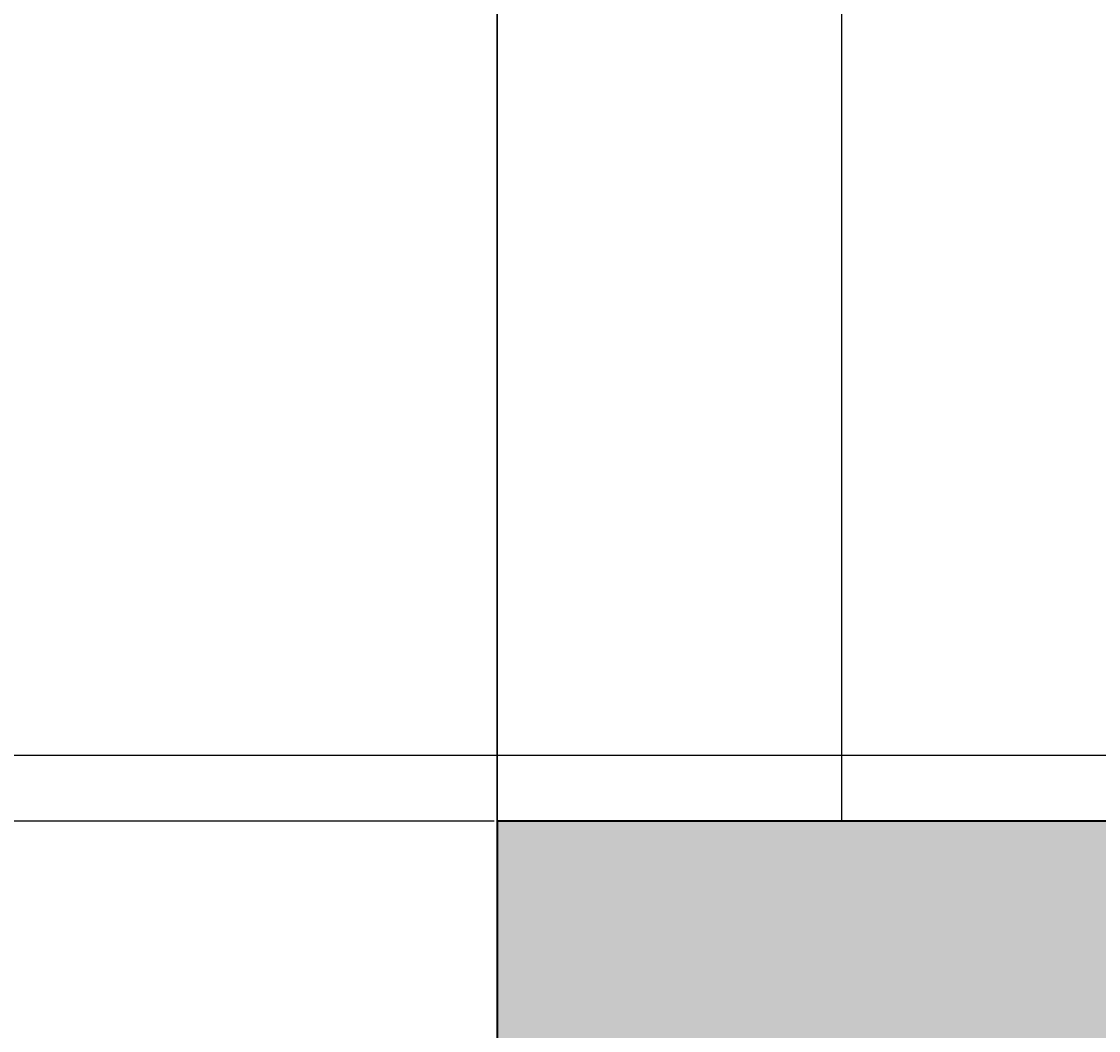
# Model space of a CAD drawing. Units: inches. Extents: x 1998 to 2588, y 1139 to 1977.
# Tile 105 of 134: x 2397 to 2422, y 1590 to 1613. Entities that reach past the tile are written whole.
import ezdxf

# ---------------------------------------------------------------- set-up
doc = ezdxf.new("R2010")
doc.units = ezdxf.units.IN
for name, color, linetype, lineweight in [('A-ANNO-DIMS', 2, 'Continuous', 18), ('A-FLOR-EVTR', 7, 'Continuous', 35), ('A-FLOR-STRS', 7, 'Continuous', 25), ('A-WALL-PATT', 252, 'Continuous', 13)]:
    doc.layers.add(name, color=color, linetype=linetype, lineweight=lineweight)
doc.styles.get("Standard").update_dxf_attribs({"font": 'arial.ttf'})
doc.dimstyles.get("Standard").update_dxf_attribs({"dimtxt": 0.18, "dimasz": 0.18, "dimexe": 0.18, "dimexo": 0.0625, "dimgap": 0.09, "dimtad": 0, "dimtih": 1, "dimtoh": 1, "dimdec": 4, "dimzin": 0, "dimdsep": 46, "dimtxsty": 'Standard', "dimcen": 0.09, "dimadec": 0, "dimazin": 0, "dimtfac": 1, "dimtdec": 4, "dimtofl": 0, "dimtmove": 0, "dimatfit": 3, "dimfxl": 1, "dimtolj": 1, "dimtzin": 0, "dimarcsym": 0})

# ---------------------------------------------------------------- blocks, each defined once
blk = doc.blocks.new('*D24')
at = {"layer": 'A-ANNO-DIMS', "color": 0, "lineweight": -2, "transparency": 16777216}
for p, q in [((2398.535, 1911.232), (2588.309, 1911.232)), ((2588.129, 1911.052), (2588.129, 1570.164)), ((2588.129, 1228.912), (2588.129, 1569.8)), ((2527.535, 1228.732), (2588.309, 1228.732))]:
    blk.add_line(p, q, dxfattribs=at)
at = {"layer": 'A-ANNO-DIMS', "color": 0, "transparency": 16777216}
for points in [[(2588.099, 1911.052), (2588.159, 1911.052), (2588.129, 1911.232)], [(2588.099, 1228.912), (2588.159, 1228.912), (2588.129, 1228.732)]]:
    blk.add_solid(points, dxfattribs=at)
at = {"layer": 'Defpoints', "color": 0, "transparency": 16777216}
for p in [(2398.473, 1911.232), (2588.129, 1911.232), (2527.473, 1228.732)]:
    blk.add_point(p, dxfattribs=at)
at = {"layer": 'A-ANNO-DIMS', "color": 0, "transparency": 16777216, "insert": (2588.129, 1569.982), "char_height": 0.18, "attachment_point": 5}
blk.add_mtext('\\A1;682.5', dxfattribs=at)
blk = doc.blocks.new('*D30')
at = {"layer": 'A-ANNO-DIMS', "color": 0, "lineweight": -2, "transparency": 16777216}
for p, q in [((2407.91, 1636.732), (1997.843, 1636.732)), ((1998.023, 1636.552), (1998.023, 1615.913)), ((1998.023, 1594.912), (1998.023, 1615.552)), ((2407.91, 1594.732), (1997.843, 1594.732))]:
    blk.add_line(p, q, dxfattribs=at)
at = {"layer": 'A-ANNO-DIMS', "color": 0, "transparency": 16777216}
for points in [[(1997.993, 1636.552), (1998.053, 1636.552), (1998.023, 1636.732)], [(1997.993, 1594.912), (1998.053, 1594.912), (1998.023, 1594.732)]]:
    blk.add_solid(points, dxfattribs=at)
at = {"layer": 'Defpoints', "color": 0, "transparency": 16777216}
for p in [(1998.023, 1636.732), (2407.973, 1636.732), (2407.973, 1594.732)]:
    blk.add_point(p, dxfattribs=at)
at = {"layer": 'A-ANNO-DIMS', "color": 0, "transparency": 16777216, "insert": (1998.023, 1615.732), "char_height": 0.18, "attachment_point": 5}
blk.add_mtext('\\A1;42', dxfattribs=at)
blk = doc.blocks.new('*D34')
at = {"layer": 'A-ANNO-DIMS', "color": 0, "lineweight": -2, "transparency": 16777216}
for p, q in [((2407.91, 1594.732), (1997.843, 1594.732)), ((1998.023, 1594.552), (1998.023, 1558.913)), ((1998.023, 1522.912), (1998.023, 1558.552)), ((2407.91, 1522.732), (1997.843, 1522.732))]:
    blk.add_line(p, q, dxfattribs=at)
at = {"layer": 'A-ANNO-DIMS', "color": 0, "transparency": 16777216}
for points in [[(1997.993, 1594.552), (1998.053, 1594.552), (1998.023, 1594.732)], [(1997.993, 1522.912), (1998.053, 1522.912), (1998.023, 1522.732)]]:
    blk.add_solid(points, dxfattribs=at)
at = {"layer": 'Defpoints', "color": 0, "transparency": 16777216}
for p in [(1998.023, 1594.732), (2407.973, 1594.732), (2407.973, 1522.732)]:
    blk.add_point(p, dxfattribs=at)
at = {"layer": 'A-ANNO-DIMS', "color": 0, "transparency": 16777216, "insert": (1998.023, 1558.732), "char_height": 0.18, "attachment_point": 5}
blk.add_mtext('\\A1;72', dxfattribs=at)
blk = doc.blocks.new('*D39')
at = {"layer": 'A-ANNO-DIMS', "color": 0, "lineweight": -2, "transparency": 16777216}
for p, q in [((2115.035, 1628.742), (2588.309, 1628.742)), ((2588.129, 1628.562), (2588.129, 1612.685)), ((2588.129, 1596.444), (2588.129, 1612.321)), ((2115.035, 1596.264), (2588.309, 1596.264))]:
    blk.add_line(p, q, dxfattribs=at)
at = {"layer": 'A-ANNO-DIMS', "color": 0, "transparency": 16777216}
for points in [[(2588.099, 1628.562), (2588.159, 1628.562), (2588.129, 1628.742)], [(2588.099, 1596.444), (2588.159, 1596.444), (2588.129, 1596.264)]]:
    blk.add_solid(points, dxfattribs=at)
at = {"layer": 'Defpoints', "color": 0, "transparency": 16777216}
for p in [(2114.973, 1628.742), (2588.129, 1628.742), (2114.973, 1596.264)]:
    blk.add_point(p, dxfattribs=at)
at = {"layer": 'A-ANNO-DIMS', "color": 0, "transparency": 16777216, "insert": (2588.129, 1612.503), "char_height": 0.18, "attachment_point": 5}
blk.add_mtext('\\A1;32.48', dxfattribs=at)
blk = doc.blocks.new('*D43')
at = {"layer": 'A-ANNO-DIMS', "color": 0, "lineweight": -2, "transparency": 16777216}
for p, q in [((2407.973, 1594.67), (2407.973, 1138.602)), ((2345.973, 1588.67), (2345.973, 1138.602)), ((2346.153, 1138.782), (2376.754, 1138.782)), ((2407.793, 1138.782), (2377.191, 1138.782))]:
    blk.add_line(p, q, dxfattribs=at)
at = {"layer": 'A-ANNO-DIMS', "color": 0, "transparency": 16777216}
for points in [[(2346.153, 1138.812), (2346.153, 1138.752), (2345.973, 1138.782)], [(2407.793, 1138.812), (2407.793, 1138.752), (2407.973, 1138.782)]]:
    blk.add_solid(points, dxfattribs=at)
at = {"layer": 'Defpoints', "color": 0, "transparency": 16777216}
for p in [(2407.973, 1594.732), (2345.973, 1588.732), (2407.973, 1138.782)]:
    blk.add_point(p, dxfattribs=at)
at = {"layer": 'A-ANNO-DIMS', "color": 0, "transparency": 16777216, "insert": (2376.973, 1138.782), "char_height": 0.18, "attachment_point": 5}
blk.add_mtext('\\A1;62', dxfattribs=at)

msp = doc.modelspace()

# ---------------------------------------------------------------- hatches: boundary and pattern name
at = {"layer": 'A-WALL-PATT'}
h = msp.add_hatch(color=256, dxfattribs=at)
h.dxf.hatch_style = 1
h.paths.add_polyline_path([(2527.4729, 1362.2324), (2510.9729, 1362.2324), (2510.9729, 1357.7324), (2518.4729, 1357.7324), (2518.4729, 1237.7324), (2503.1458, 1237.7324), (2503.1458, 1228.7324), (2527.4729, 1228.7324)])
h.paths.add_polyline_path([(2490.5682, 1362.2324), (2398.4729, 1362.2324), (2398.4729, 1357.7324), (2490.5682, 1357.7324)])
h.paths.add_polyline_path([(2224.9729, 1264.7324), (2222.9729, 1264.7324), (2222.9729, 1232.4125), (2341.4729, 1232.4125), (2341.4729, 1234.4125), (2224.9729, 1234.4125)])
h.paths.add_polyline_path([(2334.5332, 1273.7324), (2264.7638, 1273.7324), (2264.7638, 1269.5611, -0.043659), (2264.3413, 1264.7324), (2334.5332, 1264.7324)])
h.paths.add_polyline_path([(2236.9551, 1273.7324), (2234.4125, 1273.7324), (2234.4125, 1264.7324), (2236.9551, 1264.7324), (2236.9551, 1269.5611)])
h.paths.add_polyline_path([(2222.9729, 1293.2324), (2096.9729, 1293.2324), (2096.9729, 1345.0966), (2087.9729, 1345.0966), (2087.9729, 1284.2324), (2222.9729, 1284.2324), (2222.9729, 1285.137)])
h.paths.add_polyline_path([(2096.9729, 1458.7927), (2087.9729, 1458.7927), (2087.9729, 1417.7324), (2087.9729, 1413.2324), (2096.9729, 1413.2324), (2096.9729, 1417.7324)])
h.paths.add_polyline_path([(2096.9729, 1413.2324), (2087.9729, 1413.2324), (2087.9729, 1365.5012), (2096.9729, 1365.5012), (2096.9729, 1369.3358)])
h.paths.add_polyline_path([(2186.2943, 1417.7324), (2138.6074, 1417.7324), (2096.9729, 1417.7324), (2096.9729, 1413.2324), (2138.6074, 1413.2324), (2186.2943, 1413.2324)])
h.paths.add_polyline_path([(2181.4729, 1465.7324), (2176.9729, 1465.7324), (2176.9729, 1451.6434), (2181.4729, 1451.6434)])
h.paths.add_polyline_path([(2181.4729, 1422.1664), (2176.9729, 1422.1664), (2176.9729, 1417.7324), (2181.4729, 1417.7324)])
h.paths.add_polyline_path([(2063.9729, 1465.7324), (2087.9729, 1465.7324), (2087.9729, 1470.2324), (2059.4729, 1470.2324), (2059.4729, 1413.2324), (2087.9729, 1413.2324), (2087.9729, 1417.7324), (2063.9729, 1417.7324)])
h.paths.add_polyline_path([(2181.4729, 1755.2324), (2176.9729, 1755.2324), (2176.9729, 1748.6798), (2177.0513, 1748.6798), (2181.4729, 1748.6798)])
h.paths.add_polyline_path([(2227.4729, 1707.2324), (2220.4647, 1707.2324), (2220.4647, 1702.7324), (2222.9729, 1702.7324), (2222.9729, 1604.637), (2227.4729, 1604.637)])
h.paths.add_polyline_path([(2114.9729, 1702.7324), (2105.9729, 1702.7324), (2105.9729, 1628.4781, -0.0318759), (2110.1012, 1628.7416), (2114.9729, 1628.7416)])
h.paths.add_polyline_path([(2345.9729, 1739.3278), (2341.4729, 1739.3278), (2341.4729, 1647.5211), (2345.9729, 1647.5211)])
h.paths.add_polyline_path([(2350.6273, 1641.2324), (2345.9729, 1641.2324), (2345.9729, 1636.7324), (2350.6273, 1636.7324), (2350.6273, 1639.8729)])
h.paths.add_polyline_path([(2501.9729, 1641.2324), (2407.9729, 1641.2324), (2392.5005, 1641.2324), (2392.5005, 1639.8729), (2392.5005, 1636.7324), (2501.9729, 1636.7324)])
h.paths.add_polyline_path([(2510.9729, 1755.2324), (2501.9729, 1755.2324), (2501.9729, 1641.2324), (2510.9729, 1641.2324)])
h.paths.add_polyline_path([(2549.1786, 1641.2324), (2522.3775, 1641.2324), (2522.3775, 1636.7324), (2540.1786, 1636.7324), (2540.1786, 1480.7324), (2522.3775, 1480.7324), (2522.3775, 1476.2324), (2549.1786, 1476.2324)])
h.paths.add_polyline_path([(2498.1786, 1594.7324), (2407.9729, 1594.7324), (2407.9729, 1585.7324), (2416.9729, 1585.7324), (2489.1786, 1585.7324), (2489.1786, 1531.7324), (2416.9729, 1531.7324), (2407.9729, 1531.7324), (2407.9729, 1522.7324), (2498.1786, 1522.7324)])
h.paths.add_polyline_path([(2351.6437, 1480.7324), (2345.9729, 1480.7324), (2345.9729, 1476.2324), (2351.6437, 1476.2324), (2351.6437, 1477.5919)])
h.paths.add_polyline_path([(2501.9729, 1480.7324), (2498.1786, 1480.7324), (2407.9729, 1480.7324), (2393.5168, 1480.7324), (2393.5168, 1477.5919), (2393.5168, 1476.2324), (2501.9729, 1476.2324)])

# ---------------------------------------------------------------- linework, layer by layer
at = {"layer": 'A-FLOR-EVTR'}
msp.add_lwpolyline([(2407.9729, 1522.7324), (2498.1786, 1522.7324), (2498.1786, 1594.7324), (2407.9729, 1594.7324)], close=True, dxfattribs=at)
at = {"layer": 'A-FLOR-STRS'}
for p, q in [((2407.9729, 1480.7324), (2407.9729, 1636.7324)), ((2407.9729, 1636.7324), (2407.9729, 1594.7324)), ((2415.9729, 1636.7324), (2415.9729, 1594.7324)), ((2407.9729, 1594.7324), (2540.1786, 1594.7324))]:
    msp.add_line(p, q, dxfattribs=at)

# ---------------------------------------------------------------- dimensions: what is measured, and where the dimension line sits
at = {"layer": 'A-ANNO-DIMS'}
for base, p1, p2, override, picture, middle in [((2588.1286, 1911.2324), (2527.4729, 1228.7324), (2398.4729, 1911.2324), {"dimdec": 1, "dimlfac": 1, "dimrnd": 0, "dimzin": 0, "dimdsep": 46, "dimlunit": 2}, '*D24', (2588.1286, 1569.9824)), ((1998.0229, 1636.7324), (2407.9729, 1594.7324), (2407.9729, 1636.7324), {"dimdec": 0, "dimlfac": 1, "dimrnd": 0, "dimzin": 0, "dimdsep": 46, "dimlunit": 2}, '*D30', (1998.0229, 1615.7324)), ((2588.1286, 1628.7416), (2114.9729, 1596.2642), (2114.9729, 1628.7416), {"dimdec": 2, "dimlfac": 1, "dimrnd": 0, "dimzin": 0, "dimdsep": 46, "dimlunit": 2}, '*D39', (2588.1286, 1612.5029)), ((1998.0229, 1594.7324), (2407.9729, 1522.7324), (2407.9729, 1594.7324), {"dimdec": 0, "dimlfac": 1, "dimrnd": 0, "dimzin": 0, "dimdsep": 46, "dimlunit": 2}, '*D34', (1998.0229, 1558.7324))]:
    dim = msp.add_linear_dim(base=base, p1=p1, p2=p2, angle=90, dimstyle='Standard', override=override, dxfattribs=at)
    dim.commit()
    dim.dimension.update_dxf_attribs({"geometry": picture, "text_midpoint": middle})
dim = msp.add_linear_dim(base=(2407.9729, 1138.7824), p1=(2345.9729, 1588.7324), p2=(2407.9729, 1594.7324), dimstyle='Standard', override={"dimdec": 0, "dimlfac": 1, "dimrnd": 0, "dimzin": 0, "dimdsep": 46, "dimlunit": 2}, dxfattribs=at)
dim.commit()
dim.dimension.update_dxf_attribs({"geometry": '*D43', "text_midpoint": (2376.9729, 1138.7824)})

doc.saveas('drawing.dxf')
